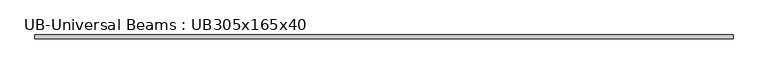
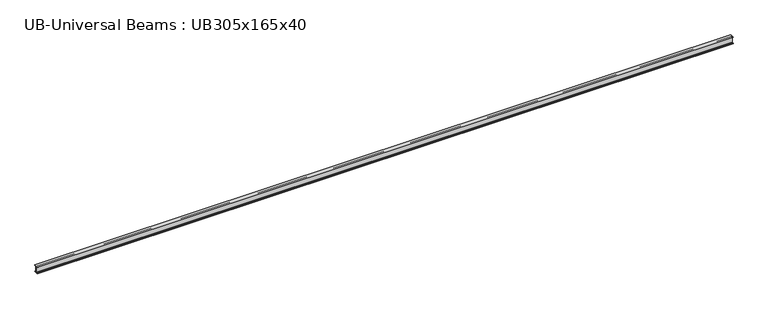
"""IFC4 building model written with IfcOpenShell, lengths in millimetres: beam geometry, UB-Universal Beams : UB305x165x40."""

from ifc_helpers import new_model, si_unit, point, frame, frame_2d, origin, place, context, project, spatial, polyline, circle_curve, trimmed, segment, composite_curve, outline, extrude, source, transform, mapped, element, save


def ub_universal_beams_ub305x165x40_be890a2c(model_context):
    return source(origin(), model_context, "Body", "SweptSolid", [
        extrude(outline(composite_curve([segment(polyline([(82.5, -141.5), (82.5, -151.7), (-82.5, -151.7), (-82.5, -141.5), (-11.9, -141.5)]), True, "CONTINUOUS"), segment(trimmed(circle_curve(frame_2d((-11.9, -132.6)), 8.9), [point((-11.9, -141.5))], [point((-3.0, -132.6))], True, "CARTESIAN"), True, "CONTINUOUS"), segment(polyline([(-3.0, -132.6), (-3.0, 132.6)]), True, "CONTINUOUS"), segment(trimmed(circle_curve(frame_2d((-11.9, 132.6)), 8.9), [point((-3.0, 132.6))], [point((-11.9, 141.5))], True, "CARTESIAN"), True, "CONTINUOUS"), segment(polyline([(-11.9, 141.5), (-82.5, 141.5), (-82.5, 151.7), (82.5, 151.7), (82.5, 141.5), (11.9, 141.5)]), True, "CONTINUOUS"), segment(trimmed(circle_curve(frame_2d((11.9, 132.6)), 8.9), [point((11.9, 141.5))], [point((3.0, 132.6))], True, "CARTESIAN"), True, "CONTINUOUS"), segment(polyline([(3.0, 132.6), (3.0, -132.6)]), True, "CONTINUOUS"), segment(trimmed(circle_curve(frame_2d((11.9, -132.6)), 8.9), [point((3.0, -132.6))], [point((11.9, -141.5))], True, "CARTESIAN"), True, "CONTINUOUS"), segment(polyline([(11.9, -141.5), (82.5, -141.5)]), True, "CONTINUOUS")], self_intersect=False)), frame((-15144.8, 0.0, 0.0), z_axis=(1.0, 0.0, 0.0), x_axis=(0.0, 1.0, 0.0)), (0.0, 0.0, 1.0), 30289.6),
    ])


if __name__ == "__main__":
    model = new_model("IFC4")
    model_context = context("Model", 3, world=origin())
    ifc_project = project(units=[si_unit("LENGTHUNIT", "METRE", prefix="MILLI")], contexts=[model_context])
    site = spatial("IfcSite", under=ifc_project)
    building = spatial("IfcBuilding", under=site)
    placement = place(None, origin())
    ub_universal_beams_ub305x165x40_shape = ub_universal_beams_ub305x165x40_be890a2c(model_context)
    element("IfcBeam", 1, ObjectType="UB-Universal Beams : UB305x165x40", at=placement, inside=building, context=model_context, shape_type="MappedRepresentation", body=[
        mapped(ub_universal_beams_ub305x165x40_shape, transform((0.0, 0.0, 0.0), x_axis=(1.0, 0.0, 0.0), y_axis=(0.0, 1.0, 0.0), z_axis=(0.0, 0.0, 1.0))),
    ])
    save(model, "model.ifc")

# Revit data of these elements
# Type "UB-Universal Beams : UB305x165x40"
#   Section Name Key = "UB305X165X40"
#   Width = 16.5 cm
#   Web Thickness = 0.6 cm
#   Web Fillet = 0.89 cm
#   Warping Constant = 164000.0 cm⁶
#   Torsional Moment of Inertia = 14.70 cm⁴
#   Section Area = 51.3 cm²
#   Plastic Modulus weak axis = 142.0 cm³
#   Plastic Modulus strong axis = 623.0 cm³
#   Nominal Weight = 40.2999 kgf/m
#   Moment of Inertia weak axis = 764.00 cm⁴
#   Moment of Inertia strong axis = 8503.00 cm⁴
#   Height = 30.34 cm
#   Flange Thickness = 1.02 cm
#   Elastic Modulus weak axis = 92.6 cm³
#   Elastic Modulus strong axis = 560.0 cm³
#   Centroid Vertical = 15.17 cm
#   Centroid Horizontal = 8.25 cm
#   Bolt Spacing = 9.0 cm
#   Length [instance default] = 1500 mm
#   Structural Material [instance default] = Metal - Steel 43-275
#   Type Comments = ""
#   Assembly Code = ""
# Element 1 (IfcBeam, "UB-Universal Beams : UB305x165x40")
#   Materials on its faces: "Metal - Steel 43-275"
# Materials
#   "Metal - Steel 43-275": class "Metal", colour RGB 247 247 247, transparency 0, Cost = 0
